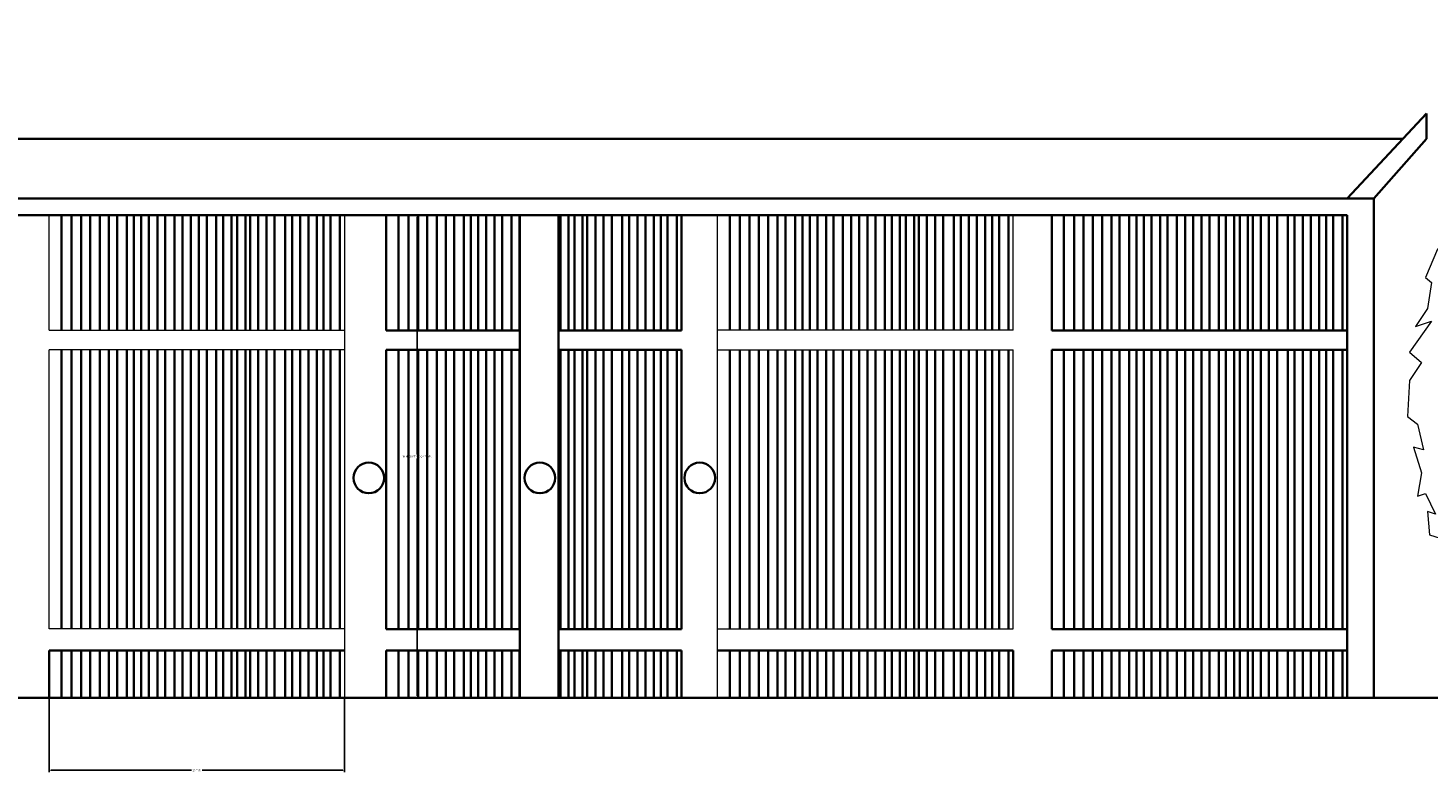
# Model space of a CAD drawing. Units: inches. Extents: x -1080 to 1950, y -1929 to 857.
# Tile 10 of 16: x 1495 to 1630, y -742 to -670. Entities that reach past the tile are written whole.
import ezdxf

# ---------------------------------------------------------------- set-up
doc = ezdxf.new("R2010")
doc.units = ezdxf.units.IN
doc.header["$MEASUREMENT"] = 0
for name, color, linetype, lineweight in [('A-ANNO-DIMS', 2, 'Continuous', 18), ('A-ELEV', 7, 'Continuous', 35), ('A-GLAZ', 4, 'Continuous', 18), ('L-PLNT', 82, 'Continuous', 13)]:
    doc.layers.add(name, color=color, linetype=linetype, lineweight=lineweight)
doc.styles.get("Standard").update_dxf_attribs({"font": 'arial.ttf'})
doc.dimstyles.get("Standard").update_dxf_attribs({"dimtxt": 0.18, "dimasz": 0.18, "dimexe": 0.18, "dimexo": 0.0625, "dimgap": 0.09, "dimtad": 0, "dimtih": 1, "dimtoh": 1, "dimdec": 4, "dimzin": 0, "dimdsep": 46, "dimtxsty": 'Standard', "dimcen": 0.09, "dimadec": 0, "dimazin": 0, "dimtfac": 1, "dimtdec": 4, "dimtofl": 0, "dimtmove": 0, "dimatfit": 3, "dimfxl": 1, "dimtolj": 1, "dimtzin": 0, "dimarcsym": 0})

# ---------------------------------------------------------------- blocks, each defined once
blk = doc.blocks.new('*U5')
blk.add_lwpolyline([(-2.754, 191.699), (-6.78, 182.851), (-13.682, 176.953), (-11.956, 173.266), (-9.656, 172.529), (-14.257, 170.317), (-13.682, 167.368), (-21.733, 157.783), (-25.184, 154.834), (-21.158, 150.41), (-21.733, 147.461), (-22.884, 140.825), (-26.334, 140.087), (-29.21, 134.926), (-28.635, 129.028), (-32.661, 128.291), (-36.111, 120.18), (-34.386, 118.706), (-35.536, 111.333), (-38.987, 106.171), (-34.386, 107.646), (-40.712, 98.798), (-37.261, 95.849), (-40.712, 90.688), (-41.287, 80.366), (-38.412, 78.154), (-36.686, 70.781), (-39.562, 71.518), (-37.261, 64.145), (-38.412, 57.509), (-36.111, 58.247), (-33.236, 52.348), (-35.536, 53.086), (-34.961, 46.45), (-30.36, 44.975), (-31.51, 36.128), (-26.334, 36.865), (-23.459, 39.814), (-18.283, 36.128), (-20.008, 33.178), (-14.832, 31.704), (-11.956, 33.178), (-12.531, 27.28), (-6.205, 22.856), (-3.905, 24.331), (0.121, 22.856), (8.173, 26.543), (11.624, 25.068), (12.199, 27.28), (21.4, 34.653), (19.675, 39.077), (23.701, 44.975), (30.027, 47.924), (30.602, 53.823), (25.426, 56.772), (32.903, 61.196), (34.053, 67.094), (30.602, 75.205), (34.628, 89.951), (26.576, 103.222), (23.701, 103.222), (28.302, 107.646), (23.701, 110.595), (26.576, 115.756), (25.426, 117.968), (20.825, 118.706), (24.276, 124.604), (22.551, 137.876), (19.1, 139.35), (22.551, 140.825), (19.675, 151.884), (14.499, 153.359), (16.224, 162.207), (12.199, 170.317), (10.473, 167.368), (5.872, 179.165), (4.147, 177.69), (0.696, 187.275), (-0.454, 185.8)], close=True)
for points in [[(-6.813, 23.669), (-6.813, 11.669), (-8.627, 0)], [(0.387, 23.669), (-0.576, 13.271), (-0.576, 3.686), (0, 0)]]:
    blk.add_lwpolyline(points)
blk = doc.blocks.new('WIN-TYPE-Q')
for p, q in [((0, 35.54), (0, 46.69)), ((28.56, 35.54), (28.56, 46.69)), ((0, 35.54), (28.56, 35.54)), ((28.56, 6.66), (28.56, 35.54)), ((0, 6.66), (0, 33.65)), ((28.56, 33.65), (0, 33.65)), ((28.56, 6.66), (0, 6.66)), ((28.56, 0), (28.56, 6.66))]:
    blk.add_line(p, q)
blk = doc.blocks.new('*D63')
at = {"layer": 'A-ANNO-DIMS', "color": 0, "lineweight": -2, "transparency": 16777216}
for p, q in [((1525.67, -688.04), (1532.79, -688.04)), ((1532.61, -688.22), (1532.61, -711.19)), ((1532.61, -734.54), (1532.61, -711.57)), ((1525.67, -734.72), (1532.79, -734.72))]:
    blk.add_line(p, q, dxfattribs=at)
at = {"layer": 'A-ANNO-DIMS', "color": 0, "transparency": 16777216}
for points in [[(1532.58, -688.22), (1532.64, -688.22), (1532.61, -688.04)], [(1532.58, -734.54), (1532.64, -734.54), (1532.61, -734.72)]]:
    blk.add_solid(points, dxfattribs=at)
at = {"layer": 'Defpoints', "color": 0, "transparency": 16777216}
for p in [(1525.6, -688.04), (1532.61, -688.04), (1525.6, -734.72)]:
    blk.add_point(p, dxfattribs=at)
at = {"layer": 'A-ANNO-DIMS', "color": 0, "transparency": 16777216, "insert": (1532.61, -711.38), "char_height": 0.18, "attachment_point": 5}
blk.add_mtext('\\A1;WINDOW TYPE Q 47 TYP.', dxfattribs=at)
blk = doc.blocks.new('*D64')
at = {"layer": 'A-ANNO-DIMS', "color": 0, "lineweight": -2, "transparency": 16777216}
for p, q in [((1497.04, -734.79), (1497.04, -741.91)), ((1525.6, -734.79), (1525.6, -741.91)), ((1497.22, -741.73), (1510.79, -741.73)), ((1525.42, -741.73), (1511.85, -741.73))]:
    blk.add_line(p, q, dxfattribs=at)
at = {"layer": 'A-ANNO-DIMS', "color": 0, "transparency": 16777216}
for points in [[(1497.22, -741.7), (1497.22, -741.76), (1497.04, -741.73)], [(1525.42, -741.7), (1525.42, -741.76), (1525.6, -741.73)]]:
    blk.add_solid(points, dxfattribs=at)
at = {"layer": 'Defpoints', "color": 0, "transparency": 16777216}
for p in [(1497.04, -734.72), (1525.6, -734.72), (1525.6, -741.73)]:
    blk.add_point(p, dxfattribs=at)
at = {"layer": 'A-ANNO-DIMS', "color": 0, "transparency": 16777216, "insert": (1511.32, -741.73), "char_height": 0.18, "attachment_point": 5}
blk.add_mtext('\\A1;29 TYP.', dxfattribs=at)

msp = doc.modelspace()

# ---------------------------------------------------------------- linework, layer by layer
at = {"layer": 'A-ELEV'}
for p, q in [((1630.14, -678.23), (1622.49, -686.45)), ((1630.14, -680.68), (1630.14, -678.23)), ((1627.86, -680.68), (1123.47, -680.68)), ((1625.05, -686.45), (1630.14, -680.68)), ((1123.47, -686.45), (1622.49, -686.45)), ((1622.49, -686.45), (1625.05, -686.45)), ((1625.05, -686.45), (1625.05, -734.72)), ((1123.47, -688.04), (1622.49, -688.04)), ((1498.24, -699.19), (1498.24, -688.04)), ((1499.21, -699.19), (1499.21, -688.04)), ((1500.13, -699.19), (1500.13, -688.04)), ((1501.01, -699.19), (1501.01, -688.04)), ((1501.94, -699.19), (1501.94, -688.04)), ((1502.82, -699.19), (1502.82, -688.04)), ((1503.61, -699.19), (1503.61, -688.04)), ((1504.54, -699.19), (1504.54, -688.04)), ((1505.24, -699.19), (1505.24, -688.04)), ((1505.95, -699.19), (1505.95, -688.04)), ((1506.69, -699.19), (1506.69, -688.04)), ((1507.53, -699.19), (1507.53, -688.04)), ((1508.25, -699.19), (1508.25, -688.04)), ((1509.15, -699.19), (1509.15, -688.04)), ((1509.94, -699.19), (1509.94, -688.04)), ((1510.73, -699.19), (1510.73, -688.04)), ((1511.51, -699.19), (1511.51, -688.04)), ((1512.3, -699.19), (1512.3, -688.04)), ((1513.2, -699.19), (1513.2, -688.04)), ((1513.88, -699.19), (1513.88, -688.04)), ((1514.67, -699.19), (1514.67, -688.04)), ((1515.23, -699.19), (1515.23, -688.04)), ((1516.02, -699.19), (1516.02, -688.04)), ((1516.47, -699.19), (1516.47, -688.04)), ((1517.26, -699.19), (1517.26, -688.04)), ((1518.05, -699.19), (1518.05, -688.04)), ((1518.84, -699.19), (1518.84, -688.04)), ((1519.86, -699.19), (1519.86, -688.04)), ((1520.53, -699.19), (1520.53, -688.04)), ((1521.32, -699.19), (1521.32, -688.04)), ((1522.11, -699.19), (1522.11, -688.04)), ((1522.9, -699.19), (1522.9, -688.04)), ((1523.57, -699.19), (1523.57, -688.04)), ((1524.25, -699.19), (1524.25, -688.04)), ((1525.15, -699.19), (1525.15, -688.04)), ((1529.62, -699.19), (1529.62, -688.04)), ((1530.81, -699.19), (1530.81, -688.04)), ((1531.78, -699.19), (1531.78, -688.04)), ((1532.7, -699.19), (1532.7, -688.04)), ((1533.58, -699.19), (1533.58, -688.04)), ((1534.51, -699.19), (1534.51, -688.04)), ((1535.39, -699.19), (1535.39, -688.04)), ((1536.18, -699.19), (1536.18, -688.04)), ((1537.11, -699.19), (1537.11, -688.04)), ((1537.81, -699.19), (1537.81, -688.04)), ((1538.52, -699.19), (1538.52, -688.04)), ((1539.27, -699.19), (1539.27, -688.04)), ((1540.1, -699.19), (1540.1, -688.04)), ((1540.82, -699.19), (1540.82, -688.04)), ((1541.72, -699.19), (1541.72, -688.04)), ((1542.51, -699.19), (1542.51, -688.04)), ((1542.52, -734.72), (1542.52, -688.04)), ((1546.27, -688.04), (1546.27, -734.72)), ((1546.45, -699.19), (1546.45, -688.04)), ((1547.24, -699.19), (1547.24, -688.04)), ((1547.81, -699.19), (1547.81, -688.04)), ((1548.59, -699.19), (1548.59, -688.04)), ((1549.04, -699.19), (1549.04, -688.04)), ((1549.83, -699.19), (1549.83, -688.04)), ((1550.62, -699.19), (1550.62, -688.04)), ((1551.41, -699.19), (1551.41, -688.04)), ((1552.43, -699.19), (1552.43, -688.04)), ((1553.1, -699.19), (1553.1, -688.04)), ((1553.89, -699.19), (1553.89, -688.04)), ((1554.68, -699.19), (1554.68, -688.04)), ((1555.47, -699.19), (1555.47, -688.04)), ((1556.15, -699.19), (1556.15, -688.04)), ((1556.82, -699.19), (1556.82, -688.04)), ((1557.72, -699.19), (1557.72, -688.04)), ((1558.17, -699.19), (1558.17, -688.04)), ((1562.84, -699.19), (1562.84, -688.04)), ((1563.81, -699.19), (1563.81, -688.04)), ((1564.74, -699.19), (1564.74, -688.04)), ((1565.62, -699.19), (1565.62, -688.04)), ((1566.54, -699.19), (1566.54, -688.04)), ((1567.42, -699.19), (1567.42, -688.04)), ((1568.22, -699.19), (1568.22, -688.04)), ((1569.14, -699.19), (1569.14, -688.04)), ((1569.85, -699.19), (1569.85, -688.04)), ((1570.55, -699.19), (1570.55, -688.04)), ((1571.3, -699.19), (1571.3, -688.04)), ((1572.14, -699.19), (1572.14, -688.04)), ((1572.85, -699.19), (1572.85, -688.04)), ((1573.75, -699.19), (1573.75, -688.04)), ((1574.54, -699.19), (1574.54, -688.04)), ((1575.33, -699.19), (1575.33, -688.04)), ((1576.12, -699.19), (1576.12, -688.04)), ((1576.91, -699.19), (1576.91, -688.04)), ((1577.81, -699.19), (1577.81, -688.04)), ((1578.49, -699.19), (1578.49, -688.04)), ((1579.27, -699.19), (1579.27, -688.04)), ((1579.84, -699.19), (1579.84, -688.04)), ((1580.63, -699.19), (1580.63, -688.04)), ((1581.08, -699.19), (1581.08, -688.04)), ((1581.87, -699.19), (1581.87, -688.04)), ((1582.66, -699.19), (1582.66, -688.04)), ((1583.44, -699.19), (1583.44, -688.04)), ((1584.46, -699.19), (1584.46, -688.04)), ((1585.14, -699.19), (1585.14, -688.04)), ((1585.92, -699.19), (1585.92, -688.04)), ((1586.71, -699.19), (1586.71, -688.04)), ((1587.5, -699.19), (1587.5, -688.04)), ((1588.18, -699.19), (1588.18, -688.04)), ((1588.86, -699.19), (1588.86, -688.04)), ((1589.76, -699.19), (1589.76, -688.04)), ((1593.93, -699.19), (1593.93, -688.04)), ((1595.12, -699.19), (1595.12, -688.04)), ((1596.09, -699.19), (1596.09, -688.04)), ((1597.02, -699.19), (1597.02, -688.04)), ((1597.9, -699.19), (1597.9, -688.04)), ((1598.82, -699.19), (1598.82, -688.04)), ((1599.7, -699.19), (1599.7, -688.04)), ((1600.49, -699.19), (1600.49, -688.04)), ((1601.42, -699.19), (1601.42, -688.04)), ((1602.12, -699.19), (1602.12, -688.04)), ((1602.83, -699.19), (1602.83, -688.04)), ((1603.58, -699.19), (1603.58, -688.04)), ((1604.41, -699.19), (1604.41, -688.04)), ((1605.13, -699.19), (1605.13, -688.04)), ((1606.03, -699.19), (1606.03, -688.04)), ((1606.82, -699.19), (1606.82, -688.04)), ((1607.61, -699.19), (1607.61, -688.04)), ((1608.4, -699.19), (1608.4, -688.04)), ((1609.19, -699.19), (1609.19, -688.04)), ((1610.09, -699.19), (1610.09, -688.04)), ((1610.76, -699.19), (1610.76, -688.04)), ((1611.55, -699.19), (1611.55, -688.04)), ((1612.12, -699.19), (1612.12, -688.04)), ((1612.9, -699.19), (1612.9, -688.04)), ((1613.36, -699.19), (1613.36, -688.04)), ((1614.14, -699.19), (1614.14, -688.04)), ((1614.93, -699.19), (1614.93, -688.04)), ((1615.72, -699.19), (1615.72, -688.04)), ((1616.74, -699.19), (1616.74, -688.04)), ((1617.41, -699.19), (1617.41, -688.04)), ((1618.2, -699.19), (1618.2, -688.04)), ((1618.99, -699.19), (1618.99, -688.04)), ((1619.78, -699.19), (1619.78, -688.04)), ((1620.46, -699.19), (1620.46, -688.04)), ((1621.13, -699.19), (1621.13, -688.04)), ((1622.03, -699.19), (1622.03, -688.04)), ((1622.49, -699.19), (1622.49, -688.04)), ((1529.62, -699.19), (1542.52, -699.19)), ((1546.27, -699.19), (1558.17, -699.19)), ((1593.93, -699.19), (1622.49, -699.19)), ((1622.49, -728.07), (1622.49, -699.19)), ((1498.24, -728.07), (1498.24, -701.07)), ((1499.21, -728.07), (1499.21, -701.07)), ((1500.13, -728.07), (1500.13, -701.07)), ((1501.01, -728.07), (1501.01, -701.07)), ((1501.94, -728.07), (1501.94, -701.07)), ((1502.82, -728.07), (1502.82, -701.07)), ((1503.61, -728.07), (1503.61, -701.07)), ((1504.54, -728.07), (1504.54, -701.07)), ((1505.24, -728.07), (1505.24, -701.07)), ((1505.95, -728.07), (1505.95, -701.07)), ((1506.69, -728.07), (1506.69, -701.07)), ((1507.53, -728.07), (1507.53, -701.07)), ((1508.25, -728.07), (1508.25, -701.07)), ((1509.15, -728.07), (1509.15, -701.07)), ((1509.94, -728.07), (1509.94, -701.07)), ((1510.73, -728.07), (1510.73, -701.07)), ((1511.51, -728.07), (1511.51, -701.07)), ((1512.3, -728.07), (1512.3, -701.07)), ((1513.2, -728.07), (1513.2, -701.07)), ((1513.88, -728.07), (1513.88, -701.07)), ((1514.67, -728.07), (1514.67, -701.07)), ((1515.23, -728.07), (1515.23, -701.07)), ((1516.02, -728.07), (1516.02, -701.07)), ((1516.47, -728.07), (1516.47, -701.07)), ((1517.26, -728.07), (1517.26, -701.07)), ((1518.05, -728.07), (1518.05, -701.07)), ((1518.84, -728.07), (1518.84, -701.07)), ((1519.86, -728.07), (1519.86, -701.07)), ((1520.53, -728.07), (1520.53, -701.07)), ((1521.32, -728.07), (1521.32, -701.07)), ((1522.11, -728.07), (1522.11, -701.07)), ((1522.9, -728.07), (1522.9, -701.07)), ((1523.57, -728.07), (1523.57, -701.07)), ((1524.25, -728.07), (1524.25, -701.07)), ((1525.15, -728.07), (1525.15, -701.07)), ((1529.62, -728.07), (1529.62, -701.07)), ((1542.52, -701.07), (1529.62, -701.07)), ((1530.81, -728.07), (1530.81, -701.07)), ((1531.78, -728.07), (1531.78, -701.07)), ((1532.7, -728.07), (1532.7, -701.07)), ((1533.58, -728.07), (1533.58, -701.07)), ((1534.51, -728.07), (1534.51, -701.07)), ((1535.39, -728.07), (1535.39, -701.07)), ((1536.18, -728.07), (1536.18, -701.07)), ((1537.11, -728.07), (1537.11, -701.07)), ((1537.81, -728.07), (1537.81, -701.07)), ((1538.52, -728.07), (1538.52, -701.07)), ((1539.27, -728.07), (1539.27, -701.07)), ((1540.1, -728.07), (1540.1, -701.07)), ((1540.82, -728.07), (1540.82, -701.07)), ((1541.72, -728.07), (1541.72, -701.07)), ((1542.51, -728.07), (1542.51, -701.07)), ((1558.17, -701.07), (1546.27, -701.07)), ((1546.45, -728.07), (1546.45, -701.07)), ((1547.24, -728.07), (1547.24, -701.07)), ((1547.81, -728.07), (1547.81, -701.07)), ((1548.59, -728.07), (1548.59, -701.07)), ((1549.04, -728.07), (1549.04, -701.07)), ((1549.83, -728.07), (1549.83, -701.07)), ((1550.62, -728.07), (1550.62, -701.07)), ((1551.41, -728.07), (1551.41, -701.07)), ((1552.43, -728.07), (1552.43, -701.07)), ((1553.1, -728.07), (1553.1, -701.07)), ((1553.89, -728.07), (1553.89, -701.07)), ((1554.68, -728.07), (1554.68, -701.07)), ((1555.47, -728.07), (1555.47, -701.07)), ((1556.15, -728.07), (1556.15, -701.07)), ((1556.82, -728.07), (1556.82, -701.07)), ((1557.72, -728.07), (1557.72, -701.07)), ((1558.17, -728.07), (1558.17, -701.07)), ((1562.84, -728.07), (1562.84, -701.07)), ((1563.81, -728.07), (1563.81, -701.07)), ((1564.74, -728.07), (1564.74, -701.07)), ((1565.62, -728.07), (1565.62, -701.07)), ((1566.54, -728.07), (1566.54, -701.07)), ((1567.42, -728.07), (1567.42, -701.07)), ((1568.22, -728.07), (1568.22, -701.07)), ((1569.14, -728.07), (1569.14, -701.07)), ((1569.85, -728.07), (1569.85, -701.07)), ((1570.55, -728.07), (1570.55, -701.07)), ((1571.3, -728.07), (1571.3, -701.07)), ((1572.14, -728.07), (1572.14, -701.07)), ((1572.85, -728.07), (1572.85, -701.07)), ((1573.75, -728.07), (1573.75, -701.07)), ((1574.54, -728.07), (1574.54, -701.07)), ((1575.33, -728.07), (1575.33, -701.07)), ((1576.12, -728.07), (1576.12, -701.07)), ((1576.91, -728.07), (1576.91, -701.07)), ((1577.81, -728.07), (1577.81, -701.07)), ((1578.49, -728.07), (1578.49, -701.07)), ((1579.27, -728.07), (1579.27, -701.07)), ((1579.84, -728.07), (1579.84, -701.07)), ((1580.63, -728.07), (1580.63, -701.07)), ((1581.08, -728.07), (1581.08, -701.07)), ((1581.87, -728.07), (1581.87, -701.07)), ((1582.66, -728.07), (1582.66, -701.07)), ((1583.44, -728.07), (1583.44, -701.07)), ((1584.46, -728.07), (1584.46, -701.07)), ((1585.14, -728.07), (1585.14, -701.07)), ((1585.92, -728.07), (1585.92, -701.07)), ((1586.71, -728.07), (1586.71, -701.07)), ((1587.5, -728.07), (1587.5, -701.07)), ((1588.18, -728.07), (1588.18, -701.07)), ((1588.86, -728.07), (1588.86, -701.07)), ((1589.76, -728.07), (1589.76, -701.07)), ((1593.93, -728.07), (1593.93, -701.07)), ((1622.49, -701.07), (1593.93, -701.07)), ((1595.12, -728.07), (1595.12, -701.07)), ((1596.09, -728.07), (1596.09, -701.07)), ((1597.02, -728.07), (1597.02, -701.07)), ((1597.9, -728.07), (1597.9, -701.07)), ((1598.82, -728.07), (1598.82, -701.07)), ((1599.7, -728.07), (1599.7, -701.07)), ((1600.49, -728.07), (1600.49, -701.07)), ((1601.42, -728.07), (1601.42, -701.07)), ((1602.12, -728.07), (1602.12, -701.07)), ((1602.83, -728.07), (1602.83, -701.07)), ((1603.58, -728.07), (1603.58, -701.07)), ((1604.41, -728.07), (1604.41, -701.07)), ((1605.13, -728.07), (1605.13, -701.07)), ((1606.03, -728.07), (1606.03, -701.07)), ((1606.82, -728.07), (1606.82, -701.07)), ((1607.61, -728.07), (1607.61, -701.07)), ((1608.4, -728.07), (1608.4, -701.07)), ((1609.19, -728.07), (1609.19, -701.07)), ((1610.09, -728.07), (1610.09, -701.07)), ((1610.76, -728.07), (1610.76, -701.07)), ((1611.55, -728.07), (1611.55, -701.07)), ((1612.12, -728.07), (1612.12, -701.07)), ((1612.9, -728.07), (1612.9, -701.07)), ((1613.36, -728.07), (1613.36, -701.07)), ((1614.14, -728.07), (1614.14, -701.07)), ((1614.93, -728.07), (1614.93, -701.07)), ((1615.72, -728.07), (1615.72, -701.07)), ((1616.74, -728.07), (1616.74, -701.07)), ((1617.41, -728.07), (1617.41, -701.07)), ((1618.2, -728.07), (1618.2, -701.07)), ((1618.99, -728.07), (1618.99, -701.07)), ((1619.78, -728.07), (1619.78, -701.07)), ((1620.46, -728.07), (1620.46, -701.07)), ((1621.13, -728.07), (1621.13, -701.07)), ((1622.03, -728.07), (1622.03, -701.07)), ((1542.52, -728.07), (1529.62, -728.07)), ((1558.17, -728.07), (1546.27, -728.07)), ((1622.49, -728.07), (1593.93, -728.07)), ((1622.49, -734.72), (1622.49, -728.07)), ((1497.04, -734.72), (1497.04, -730.16)), ((1497.04, -730.16), (1525.6, -730.16)), ((1498.24, -734.72), (1498.24, -730.16)), ((1499.21, -734.72), (1499.21, -730.16)), ((1500.13, -734.72), (1500.13, -730.16)), ((1501.01, -734.72), (1501.01, -730.16)), ((1501.94, -734.72), (1501.94, -730.16)), ((1502.82, -734.72), (1502.82, -730.16)), ((1503.61, -734.72), (1503.61, -730.16)), ((1504.54, -734.72), (1504.54, -730.16)), ((1505.24, -734.72), (1505.24, -730.16)), ((1505.95, -734.72), (1505.95, -730.16)), ((1506.69, -734.72), (1506.69, -730.16)), ((1507.53, -734.72), (1507.53, -730.16)), ((1508.25, -734.72), (1508.25, -730.16)), ((1509.15, -734.72), (1509.15, -730.16)), ((1509.94, -734.72), (1509.94, -730.16)), ((1510.73, -734.72), (1510.73, -730.16)), ((1511.51, -734.72), (1511.51, -730.16)), ((1512.3, -734.72), (1512.3, -730.16)), ((1513.2, -734.72), (1513.2, -730.16)), ((1513.88, -734.72), (1513.88, -730.16)), ((1514.67, -734.72), (1514.67, -730.16)), ((1515.23, -734.72), (1515.23, -730.16)), ((1516.02, -734.72), (1516.02, -730.16)), ((1516.47, -734.72), (1516.47, -730.16)), ((1517.26, -734.72), (1517.26, -730.16)), ((1518.05, -734.72), (1518.05, -730.16)), ((1518.84, -734.72), (1518.84, -730.16)), ((1519.86, -734.72), (1519.86, -730.16)), ((1520.53, -734.72), (1520.53, -730.16)), ((1521.32, -734.72), (1521.32, -730.16)), ((1522.11, -734.72), (1522.11, -730.16)), ((1522.9, -734.72), (1522.9, -730.16)), ((1523.57, -734.72), (1523.57, -730.16)), ((1524.25, -734.72), (1524.25, -730.16)), ((1525.15, -734.72), (1525.15, -730.16)), ((1529.62, -734.72), (1529.62, -730.16)), ((1529.62, -730.16), (1542.52, -730.16)), ((1530.81, -734.72), (1530.81, -730.16)), ((1531.78, -734.72), (1531.78, -730.16)), ((1532.7, -734.72), (1532.7, -730.16)), ((1533.58, -734.72), (1533.58, -730.16)), ((1534.51, -734.72), (1534.51, -730.16)), ((1535.39, -734.72), (1535.39, -730.16)), ((1536.18, -734.72), (1536.18, -730.16)), ((1537.11, -734.72), (1537.11, -730.16)), ((1537.81, -734.72), (1537.81, -730.16)), ((1538.52, -734.72), (1538.52, -730.16)), ((1539.27, -734.72), (1539.27, -730.16)), ((1540.1, -734.72), (1540.1, -730.16)), ((1540.82, -734.72), (1540.82, -730.16)), ((1541.72, -734.72), (1541.72, -730.16)), ((1542.51, -734.72), (1542.51, -730.16)), ((1546.27, -730.16), (1558.17, -730.16)), ((1546.45, -734.72), (1546.45, -730.16)), ((1547.24, -734.72), (1547.24, -730.16)), ((1547.81, -734.72), (1547.81, -730.16)), ((1548.59, -734.72), (1548.59, -730.16)), ((1549.04, -734.72), (1549.04, -730.16)), ((1549.83, -734.72), (1549.83, -730.16)), ((1550.62, -734.72), (1550.62, -730.16)), ((1551.41, -734.72), (1551.41, -730.16)), ((1552.43, -734.72), (1552.43, -730.16)), ((1553.1, -734.72), (1553.1, -730.16)), ((1553.89, -734.72), (1553.89, -730.16)), ((1554.68, -734.72), (1554.68, -730.16)), ((1555.47, -734.72), (1555.47, -730.16)), ((1556.15, -734.72), (1556.15, -730.16)), ((1556.82, -734.72), (1556.82, -730.16)), ((1557.72, -734.72), (1557.72, -730.16)), ((1558.17, -734.72), (1558.17, -730.16)), ((1561.65, -730.16), (1590.21, -730.16)), ((1562.84, -734.72), (1562.84, -730.16)), ((1563.81, -734.72), (1563.81, -730.16)), ((1564.74, -734.72), (1564.74, -730.16)), ((1565.62, -734.72), (1565.62, -730.16)), ((1566.54, -734.72), (1566.54, -730.16)), ((1567.42, -734.72), (1567.42, -730.16)), ((1568.22, -734.72), (1568.22, -730.16)), ((1569.14, -734.72), (1569.14, -730.16)), ((1569.85, -734.72), (1569.85, -730.16)), ((1570.55, -734.72), (1570.55, -730.16)), ((1571.3, -734.72), (1571.3, -730.16)), ((1572.14, -734.72), (1572.14, -730.16)), ((1572.85, -734.72), (1572.85, -730.16)), ((1573.75, -734.72), (1573.75, -730.16)), ((1574.54, -734.72), (1574.54, -730.16)), ((1575.33, -734.72), (1575.33, -730.16)), ((1576.12, -734.72), (1576.12, -730.16)), ((1576.91, -734.72), (1576.91, -730.16)), ((1577.81, -734.72), (1577.81, -730.16)), ((1578.49, -734.72), (1578.49, -730.16)), ((1579.27, -734.72), (1579.27, -730.16)), ((1579.84, -734.72), (1579.84, -730.16)), ((1580.63, -734.72), (1580.63, -730.16)), ((1581.08, -734.72), (1581.08, -730.16)), ((1581.87, -734.72), (1581.87, -730.16)), ((1582.66, -734.72), (1582.66, -730.16)), ((1583.44, -734.72), (1583.44, -730.16)), ((1584.46, -734.72), (1584.46, -730.16)), ((1585.14, -734.72), (1585.14, -730.16)), ((1585.92, -734.72), (1585.92, -730.16)), ((1586.71, -734.72), (1586.71, -730.16)), ((1587.5, -734.72), (1587.5, -730.16)), ((1588.18, -734.72), (1588.18, -730.16)), ((1588.86, -734.72), (1588.86, -730.16)), ((1589.76, -734.72), (1589.76, -730.16)), ((1590.21, -734.72), (1590.21, -730.16)), ((1593.93, -734.72), (1593.93, -730.16)), ((1593.93, -730.16), (1622.49, -730.16)), ((1595.12, -734.72), (1595.12, -730.16)), ((1596.09, -734.72), (1596.09, -730.16)), ((1597.02, -734.72), (1597.02, -730.16)), ((1597.9, -734.72), (1597.9, -730.16)), ((1598.82, -734.72), (1598.82, -730.16)), ((1599.7, -734.72), (1599.7, -730.16)), ((1600.49, -734.72), (1600.49, -730.16)), ((1601.42, -734.72), (1601.42, -730.16)), ((1602.12, -734.72), (1602.12, -730.16)), ((1602.83, -734.72), (1602.83, -730.16)), ((1603.58, -734.72), (1603.58, -730.16)), ((1604.41, -734.72), (1604.41, -730.16)), ((1605.13, -734.72), (1605.13, -730.16)), ((1606.03, -734.72), (1606.03, -730.16)), ((1606.82, -734.72), (1606.82, -730.16)), ((1607.61, -734.72), (1607.61, -730.16)), ((1608.4, -734.72), (1608.4, -730.16)), ((1609.19, -734.72), (1609.19, -730.16)), ((1610.09, -734.72), (1610.09, -730.16)), ((1610.76, -734.72), (1610.76, -730.16)), ((1611.55, -734.72), (1611.55, -730.16)), ((1612.12, -734.72), (1612.12, -730.16)), ((1612.9, -734.72), (1612.9, -730.16)), ((1613.36, -734.72), (1613.36, -730.16)), ((1614.14, -734.72), (1614.14, -730.16)), ((1614.93, -734.72), (1614.93, -730.16)), ((1615.72, -734.72), (1615.72, -730.16)), ((1616.74, -734.72), (1616.74, -730.16)), ((1617.41, -734.72), (1617.41, -730.16)), ((1618.2, -734.72), (1618.2, -730.16)), ((1618.99, -734.72), (1618.99, -730.16)), ((1619.78, -734.72), (1619.78, -730.16)), ((1620.46, -734.72), (1620.46, -730.16)), ((1621.13, -734.72), (1621.13, -730.16)), ((1622.03, -734.72), (1622.03, -730.16)), ((1442.74, -734.72), (1691.4, -734.72))]:
    msp.add_line(p, q, dxfattribs=at)
for centre in [(1527.94, -713.46), (1544.47, -713.46), (1559.92, -713.46)]:
    msp.add_circle(centre, 1.48, dxfattribs=at)

# ---------------------------------------------------------------- block references
at = {"layer": 'A-GLAZ'}
msp.add_blockref('WIN-TYPE-Q', (1497.05, -734.72), dxfattribs=at)
at = {"layer": 'A-GLAZ', "extrusion": (0, 0, -1), "zscale": -1}
msp.add_blockref('WIN-TYPE-Q', (-1590.21, -734.72), dxfattribs=at)
at = {"layer": 'L-PLNT', "xscale": 0.3373382957572102, "yscale": 0.3373382957572102, "zscale": 0.3373382957572102}
msp.add_blockref('*U5', (1642.24, -734.62), dxfattribs=at)

# ---------------------------------------------------------------- dimensions: what is measured, and where the dimension line sits
at = {"layer": 'A-ANNO-DIMS'}
dim = msp.add_linear_dim(base=(1532.61, -688.04), p1=(1525.6, -734.72), p2=(1525.6, -688.04), angle=90, text='WINDOW TYPE Q <> TYP.', dimstyle='Standard', override={"dimdec": 0, "dimlfac": 1, "dimrnd": 0, "dimzin": 0, "dimdsep": 46, "dimlunit": 2}, dxfattribs=at)
dim.commit()
dim.dimension.update_dxf_attribs({"geometry": '*D63', "text_midpoint": (1532.61, -711.38)})
dim = msp.add_linear_dim(base=(1525.6, -741.73), p1=(1497.04, -734.72), p2=(1525.6, -734.72), text='<> TYP.', dimstyle='Standard', override={"dimdec": 0, "dimlfac": 1, "dimrnd": 0, "dimzin": 0, "dimdsep": 46, "dimlunit": 2}, dxfattribs=at)
dim.commit()
dim.dimension.update_dxf_attribs({"geometry": '*D64', "text_midpoint": (1511.32, -741.73)})

doc.saveas('drawing.dxf')
